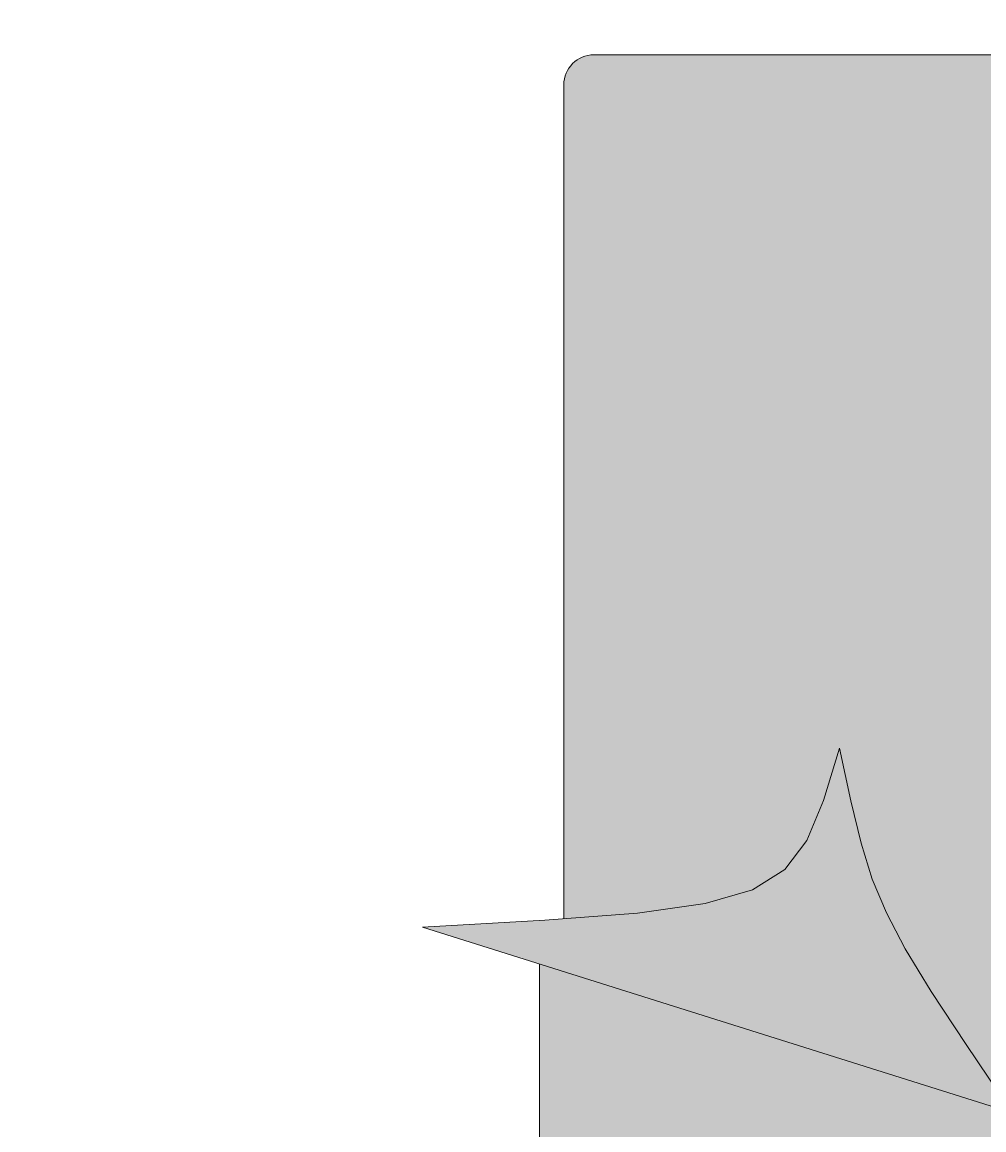
# Model space of a CAD drawing. Units: millimetres. Extents: x 27017497 to 27018854, y 7058029 to 7059154.
# Tile 22 of 91: x 27017651 to 27017702, y 7058163 to 7058222. Entities that reach past the tile are written whole.
import ezdxf

# ---------------------------------------------------------------- set-up
doc = ezdxf.new("R2010")
doc.units = ezdxf.units.MM
doc.layers.add('A-ANNO-DIMS', color=2, linetype='Continuous', lineweight=18)
doc.layers.add('A-FURN', color=8, linetype='Continuous', lineweight=18)
doc.layers.add('A-FURN-PATT', color=177, linetype='Continuous', lineweight=13, true_color=0x293189)
doc.styles.get("Standard").update_dxf_attribs({"font": 'arial.ttf'})
doc.dimstyles.get("Standard").update_dxf_attribs({"dimtxt": 0.18, "dimasz": 0.18, "dimexe": 0.18, "dimexo": 0.0625, "dimgap": 0.09, "dimtad": 0, "dimtih": 1, "dimtoh": 1, "dimdec": 4, "dimzin": 0, "dimdsep": 46, "dimtxsty": 'Standard', "dimcen": 0.09, "dimadec": 0, "dimazin": 0, "dimtfac": 1, "dimtdec": 4, "dimtofl": 0, "dimtmove": 0, "dimatfit": 3, "dimfxl": 1, "dimtolj": 1, "dimtzin": 0, "dimarcsym": 0})

# ---------------------------------------------------------------- blocks, each defined once
blk = doc.blocks.new('CAMMAT')
for p, q in [((0.6826, -0.5169), (0.6826, -0.7603)), ((0.0535, -0.5623), (0.8382, -0.8093)), ((0.65, -0.8204), (0.65, -1.93)), ((0.61, -1.97), (-0.61, -1.97))]:
    blk.add_line(p, q)
for points in [[(0.2832, -1.0476), (0.2681, -0.9772), (0.2545, -0.921), (0.2396, -0.8732), (0.2209, -0.8282), (0.1957, -0.7803), (0.1611, -0.7238), (0.1147, -0.653), (0.0535, -0.5623)], [(0.8382, -0.8093), (0.6753, -0.8185), (0.5522, -0.828), (0.4622, -0.8406), (0.399, -0.8591), (0.356, -0.8862), (0.3267, -0.9248), (0.3046, -0.9777), (0.2832, -1.0476)]]:
    blk.add_lwpolyline(points)
blk.add_arc((0.61, -1.93), 0.04, 270, 360)
blk = doc.blocks.new('*D47')
at = {"layer": 'A-ANNO-DIMS', "color": 0, "lineweight": -2, "transparency": 16777216}
for p, q in [((27017561.166, 7058294.35), (27017561.166, 7058028.6)), ((27018790.606, 7058294.35), (27018790.606, 7058028.6)), ((27017561.346, 7058028.78), (27018175.431, 7058028.78)), ((27018790.426, 7058028.78), (27018176.341, 7058028.78))]:
    blk.add_line(p, q, dxfattribs=at)
at = {"layer": 'A-ANNO-DIMS', "color": 0, "transparency": 16777216}
for points in [[(27017561.346, 7058028.81), (27017561.346, 7058028.75), (27017561.166, 7058028.78)], [(27018790.426, 7058028.81), (27018790.426, 7058028.75), (27018790.606, 7058028.78)]]:
    blk.add_solid(points, dxfattribs=at)
at = {"layer": 'Defpoints', "color": 0, "transparency": 16777216}
for p in [(27017561.166, 7058294.412), (27018790.606, 7058294.412), (27018790.606, 7058028.78)]:
    blk.add_point(p, dxfattribs=at)
at = {"layer": 'A-ANNO-DIMS', "color": 0, "transparency": 16777216, "insert": (27018175.886, 7058028.78), "char_height": 0.18, "attachment_point": 5}
blk.add_mtext('\\A1;1229.4', dxfattribs=at)
blk = doc.blocks.new('*D48')
at = {"layer": 'A-ANNO-DIMS', "color": 0, "lineweight": -2, "transparency": 16777216}
for p, q in [((27018463.498, 7058622.912), (27017497.536, 7058622.912)), ((27017497.716, 7058622.732), (27017497.716, 7058357.753)), ((27017497.716, 7058092.41), (27017497.716, 7058357.389)), ((27018555.129, 7058092.23), (27017497.536, 7058092.23))]:
    blk.add_line(p, q, dxfattribs=at)
at = {"layer": 'A-ANNO-DIMS', "color": 0, "transparency": 16777216}
for points in [[(27017497.686, 7058622.732), (27017497.746, 7058622.732), (27017497.716, 7058622.912)], [(27017497.686, 7058092.41), (27017497.746, 7058092.41), (27017497.716, 7058092.23)]]:
    blk.add_solid(points, dxfattribs=at)
at = {"layer": 'Defpoints', "color": 0, "transparency": 16777216}
for p in [(27018463.561, 7058622.912), (27017497.716, 7058092.23), (27018555.192, 7058092.23)]:
    blk.add_point(p, dxfattribs=at)
at = {"layer": 'A-ANNO-DIMS', "color": 0, "transparency": 16777216, "insert": (27017497.716, 7058357.571), "char_height": 0.18, "attachment_point": 5}
blk.add_mtext('\\A1;530.7', dxfattribs=at)

msp = doc.modelspace()

# ---------------------------------------------------------------- hatches: boundary and pattern name
at = {"layer": 'A-FURN-PATT'}
h = msp.add_hatch(color=256, dxfattribs=at)
h.dxf.hatch_style = 1
h.paths.add_polyline_path([(27017731.53, 7058218.852, 0.414214), (27017729.937, 7058220.445), (27017681.344, 7058220.445, 0.414214), (27017679.751, 7058218.852), (27017679.751, 7058174.658), (27017683.647, 7058174.959), (27017687.23, 7058175.46), (27017689.748, 7058176.196), (27017691.461, 7058177.277), (27017692.628, 7058178.816), (27017693.508, 7058180.922), (27017694.36, 7058183.707), (27017694.963, 7058180.902), (27017695.506, 7058178.662), (27017696.096, 7058176.759), (27017696.84, 7058174.966), (27017697.847, 7058173.059), (27017699.222, 7058170.809), (27017701.073, 7058167.99), (27017703.508, 7058164.376), (27017705.943, 7058167.99), (27017707.794, 7058170.809), (27017709.169, 7058173.059), (27017710.176, 7058174.966), (27017710.92, 7058176.759), (27017711.51, 7058178.662), (27017712.053, 7058180.902), (27017712.656, 7058183.707), (27017713.508, 7058180.922), (27017714.388, 7058178.816), (27017715.555, 7058177.277), (27017717.268, 7058176.196), (27017719.786, 7058175.46), (27017723.369, 7058174.959), (27017728.274, 7058174.58), (27017731.53, 7058174.396)])
h.paths.add_polyline_path([(27017723.369, 7058174.959), (27017719.786, 7058175.46), (27017717.268, 7058176.196), (27017715.555, 7058177.277), (27017714.388, 7058178.816), (27017713.508, 7058180.922), (27017712.656, 7058183.707), (27017712.053, 7058180.902), (27017711.51, 7058178.662), (27017710.92, 7058176.759), (27017710.176, 7058174.966), (27017709.169, 7058173.059), (27017707.794, 7058170.809), (27017705.943, 7058167.99), (27017703.508, 7058164.376), (27017734.763, 7058174.214), (27017728.274, 7058174.58)])
h.paths.add_polyline_path([(27017696.84, 7058174.966), (27017696.096, 7058176.759), (27017695.506, 7058178.662), (27017694.963, 7058180.902), (27017694.36, 7058183.707), (27017693.508, 7058180.922), (27017692.628, 7058178.816), (27017691.461, 7058177.277), (27017689.748, 7058176.196), (27017687.23, 7058175.46), (27017683.647, 7058174.959), (27017679.751, 7058174.658), (27017678.741, 7058174.58), (27017672.253, 7058174.214), (27017703.508, 7058164.376), (27017701.073, 7058167.99), (27017699.222, 7058170.809), (27017697.847, 7058173.059)])
h.paths.add_polyline_path([(27017678.454, 7058172.262), (27017678.454, 7058162.569), (27017733.139, 7058162.569), (27017733.139, 7058173.703), (27017703.508, 7058164.376)])
h.paths.add_polyline_path([(27017730.145, 7058158.291, 0.41419), (27017728.95, 7058159.485), (27017707.491, 7058159.485, 0.414214), (27017706.296, 7058158.29), (27017706.296, 7058148.731, 0.414214), (27017707.491, 7058147.536), (27017728.95, 7058147.536, 0.414237), (27017730.145, 7058148.731)], flags=0)
h.paths.add_polyline_path([(27017731.53, 7058162.569), (27017679.751, 7058162.569), (27017679.751, 7058146.361, 0.414214), (27017681.344, 7058144.768), (27017729.937, 7058144.768, 0.414214), (27017731.53, 7058146.361)])
h.paths.add_polyline_path([(27017703.354, 7058159.485, -0.41419), (27017704.549, 7058158.291), (27017704.549, 7058148.731, -0.414237), (27017703.354, 7058147.536), (27017681.894, 7058147.536, -0.41419), (27017680.699, 7058148.731), (27017680.699, 7058158.29, -0.414237), (27017681.894, 7058159.485)], flags=0)
h.paths.add_polyline_path([(27017707.491, 7058159.485), (27017728.95, 7058159.485, -0.41419), (27017730.145, 7058158.291), (27017730.145, 7058148.731, -0.414237), (27017728.95, 7058147.536), (27017707.491, 7058147.536, -0.414214), (27017706.296, 7058148.731), (27017706.296, 7058158.29, -0.414214)], flags=16)
h.paths.add_polyline_path([(27017704.549, 7058158.291, 0.41419), (27017703.354, 7058159.485), (27017681.894, 7058159.485, 0.414237), (27017680.699, 7058158.29), (27017680.699, 7058148.731, 0.41419), (27017681.894, 7058147.536), (27017703.354, 7058147.536, 0.414237), (27017704.549, 7058148.731)], flags=16)
h.paths.add_polyline_path([(27017752.64, 7058160.7), (27017732.725, 7058160.7), (27017732.725, 7058144.768), (27017752.64, 7058144.768)])
h.paths.add_polyline_path([(27017748.698, 7058152.101, -1), (27017736.749, 7058152.101, -1)], flags=16)
h.paths.add_polyline_path([(27017746.424, 7058152.101, -1), (27017739.024, 7058152.101, -1)], flags=0)
h.paths.add_polyline_path([(27017678.556, 7058160.7), (27017658.641, 7058160.7), (27017658.641, 7058144.768), (27017678.556, 7058144.768)])
h.paths.add_polyline_path([(27017674.806, 7058152.101, -1), (27017662.857, 7058152.101, -1)], flags=16)
h.paths.add_polyline_path([(27017672.531, 7058152.101, -1), (27017665.131, 7058152.101, -1)], flags=0)

# ---------------------------------------------------------------- block references
at = {"layer": 'A-FURN', "xscale": 39.82996475819422, "yscale": 39.82996475819422, "zscale": 39.82996475819422, "rotation": 180}
msp.add_blockref('CAMMAT', (27017705.64, 7058141.98), dxfattribs=at)

# ---------------------------------------------------------------- dimensions: what is measured, and where the dimension line sits
at = {"layer": 'A-ANNO-DIMS'}
dim = msp.add_linear_dim(base=(27017497.716, 7058092.23), p1=(27018463.561, 7058622.912), p2=(27018555.192, 7058092.23), angle=90, dimstyle='Standard', override={"dimdec": 1, "dimlfac": 1, "dimrnd": 0, "dimzin": 0, "dimdsep": 46, "dimlunit": 2}, dxfattribs=at)
dim.commit()
dim.dimension.update_dxf_attribs({"geometry": '*D48', "text_midpoint": (27017497.716, 7058357.571)})
dim = msp.add_linear_dim(base=(27018790.606, 7058028.78), p1=(27017561.166, 7058294.412), p2=(27018790.606, 7058294.412), dimstyle='Standard', override={"dimdec": 1, "dimlfac": 1, "dimrnd": 0, "dimzin": 0, "dimdsep": 46, "dimlunit": 2}, dxfattribs=at)
dim.commit()
dim.dimension.update_dxf_attribs({"geometry": '*D47', "text_midpoint": (27018175.886, 7058028.78)})

doc.saveas('drawing.dxf')
